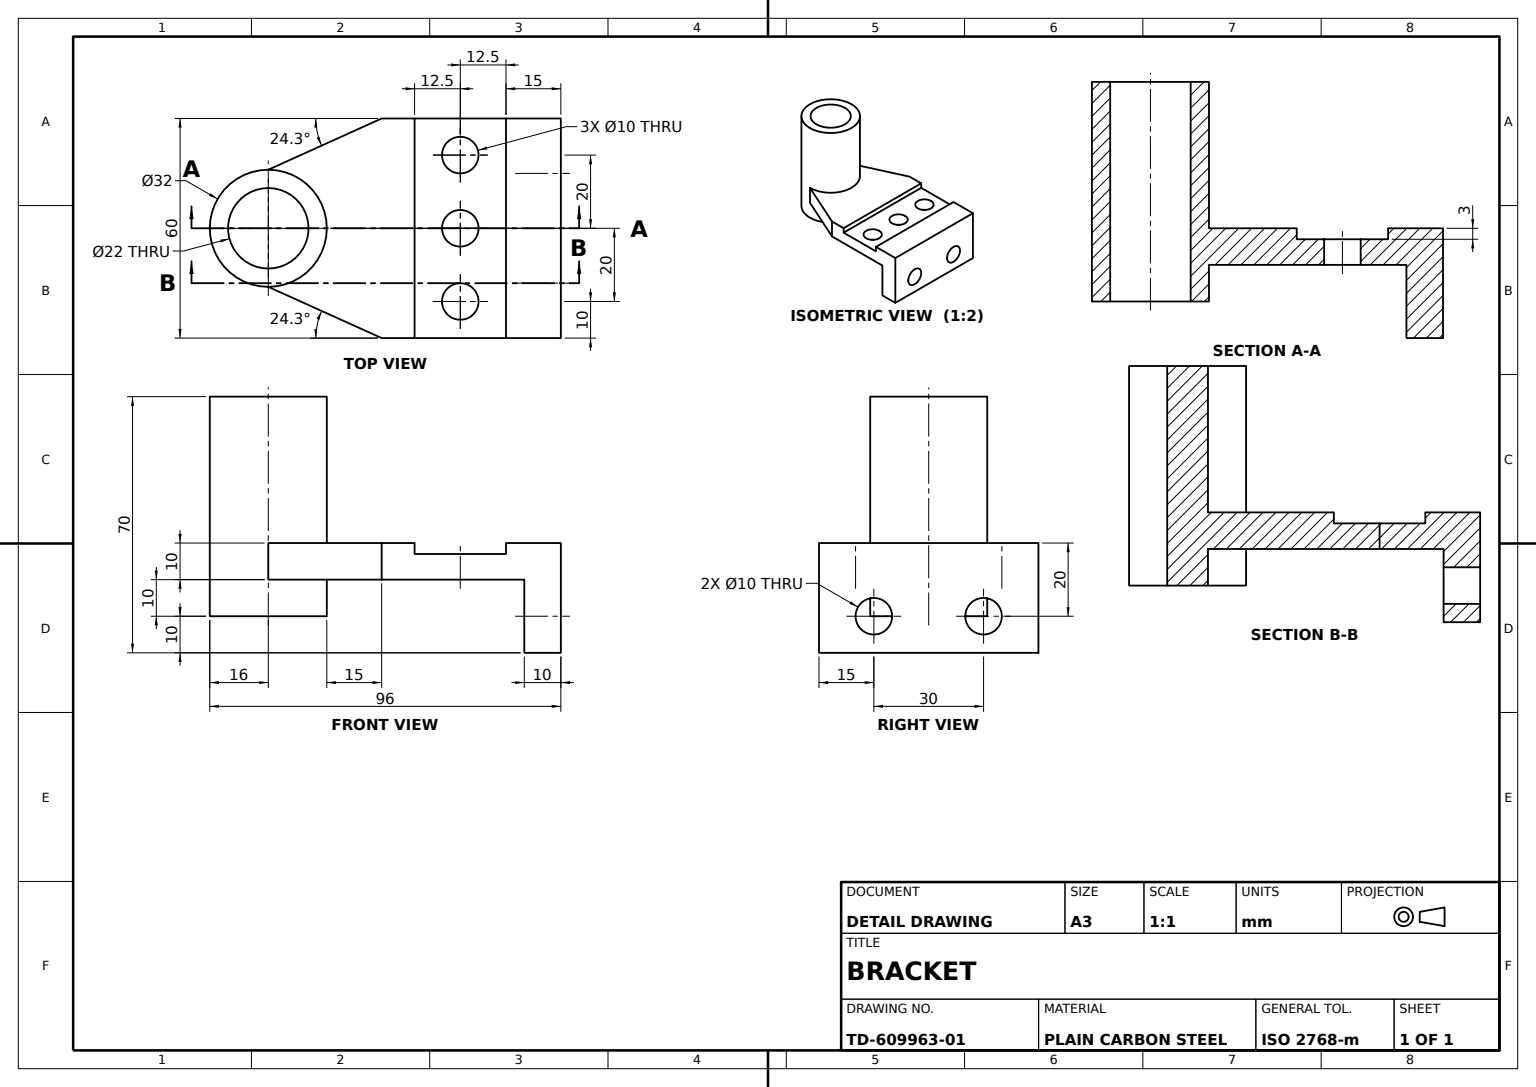
from build123d import *

# Parameters (mm, degrees)
BRACKET_BODY_60MM_DEPTH      = 30
TOP_HOLES_SKETCH_R           = 5
TOP_HOLES_DEPTH              = 15
TOP_GROOVE_CUT_DEPTH         = 15
HINGE_TUBE_UPPER_SKETCH_R    = 16
HINGE_TUBE_UPPER_SKETCH_R_2  = 11
HINGE_TUBE_UPPER_32X40_DEPTH = 40
HINGE_START                  = -20
HINGE_TUBE_LOWER_SKETCH_R    = 16
HINGE_TUBE_LOWER_SKETCH_R_2  = 11
HINGE_TUBE_LOWER_32X20_DEPTH = 20
HINGE_BORE_SKETCH_R          = 11
HINGE_BORE_22_DEPTH          = 20
SIDE_HOLES_SKETCH_R          = 5
SIDE_HOLES_DEPTH             = 20


with BuildPart() as part:
    # Bracket Profile Sketch → Bracket Body 60mm (new, symmetric)
    with BuildSketch(Plane.XY):
        Polygon((0, 0), (70, 0), (70, -20), (80, -20), (80, 10), (65, 10), (65, 7), (40, 7), (40, 10), (0, 10), align=None)
    extrude(amount=BRACKET_BODY_60MM_DEPTH, both=True)

    # Top Holes Sketch → Top Holes (cut)
    with BuildSketch(Plane(origin=(80, 0, 0), x_dir=(0, 0, -1), z_dir=(1, 0, 0))):
        with Locations((-15, -10)):
            Circle(TOP_HOLES_SKETCH_R)
        with Locations((15, -10)):
            Circle(TOP_HOLES_SKETCH_R)
    extrude(amount=-TOP_HOLES_DEPTH, mode=Mode.SUBTRACT)

    # Top Groove Sketch → Top Groove Cut (cut)
    with BuildSketch(Plane(origin=(0, 10, 0), x_dir=(1, 0, 0), z_dir=(0, 1, 0))):
        Polygon((0, 16), (31, 30), (0, 30), align=None)
        Polygon((31, -30), (0, -16), (0, -30), align=None)
    extrude(amount=-TOP_GROOVE_CUT_DEPTH, mode=Mode.SUBTRACT)

    # Hinge Tube Upper Sketch → Hinge Tube Upper Ø32x40 (add)
    with BuildSketch(Plane(origin=(0, 10, 0), x_dir=(1, 0, 0), z_dir=(0, 1, 0))):
        with Locations(Location((0, 0, 0), (0, 0, 270))):
            Circle(HINGE_TUBE_UPPER_SKETCH_R)
        with Locations(Location((0, 0, 0), (0, 0, 270))):
            Circle(HINGE_TUBE_UPPER_SKETCH_R_2, mode=Mode.SUBTRACT)
    extrude(amount=HINGE_TUBE_UPPER_32X40_DEPTH)

    # Hinge Tube Lower Sketch → Hinge Tube Lower Ø32x20 (add)
    with BuildSketch(Plane(origin=(0, 10, 0), x_dir=(1, 0, 0), z_dir=(0, 1, 0)).offset(HINGE_START)):
        with Locations(Location((0, 0, 0), (0, 0, 270))):
            Circle(HINGE_TUBE_LOWER_SKETCH_R)
        with Locations(Location((0, 0, 0), (0, 0, 270))):
            Circle(HINGE_TUBE_LOWER_SKETCH_R_2, mode=Mode.SUBTRACT)
    extrude(amount=HINGE_TUBE_LOWER_32X20_DEPTH)

    # Hinge Bore Sketch → Hinge Bore Ø22 (cut)
    with BuildSketch(Plane(origin=(0, 10, 0), x_dir=(1, 0, 0), z_dir=(0, 1, 0)).offset(HINGE_START)):
        with Locations(Location((0, 0, 0), (0, 0, 270))):
            Circle(HINGE_BORE_SKETCH_R)
    extrude(amount=HINGE_BORE_22_DEPTH, mode=Mode.SUBTRACT)

    # Side Holes Sketch → Side Holes (cut)
    with BuildSketch(Plane(origin=(0, 7, 0), x_dir=(1, 0, 0), z_dir=(0, 1, 0))):
        with Locations(Location((52.5, -20, 0), (0, 0, 270))):
            Circle(SIDE_HOLES_SKETCH_R)
        with Locations(Location((52.5, 0, 0), (0, 0, 270))):
            Circle(SIDE_HOLES_SKETCH_R)
        with Locations(Location((52.5, 20, 0), (0, 0, 270))):
            Circle(SIDE_HOLES_SKETCH_R)
    extrude(amount=-SIDE_HOLES_DEPTH, mode=Mode.SUBTRACT)


solid = part.part
